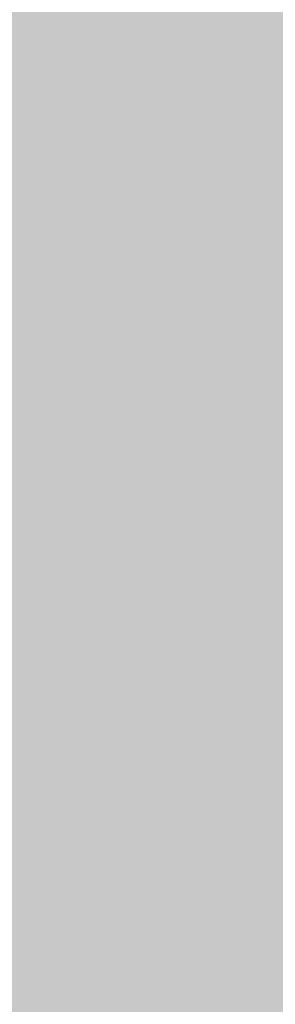
# Model space of a CAD drawing. Units: inches. Extents: x 2083 to 3317, y 1141 to 2115.
# Tile 216 of 256: x 3126.132 to 3126.67, y 1265.165 to 1267.234. Entities that reach past the tile are written whole.
import ezdxf

# ---------------------------------------------------------------- set-up
doc = ezdxf.new("R2010")
doc.units = ezdxf.units.IN
doc.layers.add('A-ANNO-DIMS', color=2, linetype='Continuous', lineweight=18)
doc.layers.add('A-WALL-PATT', color=251, linetype='Continuous', lineweight=13, true_color=0x636466)
doc.styles.get("Standard").update_dxf_attribs({"font": 'arial.ttf'})
doc.dimstyles.new('ISO-25', dxfattribs={"dimtxt": 12, "dimasz": 12, "dimexe": 1.25, "dimexo": 0.625, "dimtad": 1, "dimlunit": 3, "dimtxsty": 'Standard', "dimcen": 2.5, "dimadec": 0, "dimazin": 0, "dimtfac": 1, "dimtmove": 0, "dimatfit": 3, "dimfxl": 1, "dimarcsym": 0})

# ---------------------------------------------------------------- blocks, each defined once
blk = doc.blocks.new('*D26')
at = {"layer": 'A-ANNO-DIMS', "color": 0, "lineweight": -2, "transparency": 16777216}
for p, q in [((3088.9858, 1274.9151), (3088.9858, 1270.952)), ((3111.24, 1274.9151), (3111.24, 1270.952)), ((3076.9858, 1272.202), (2840.2624, 1272.202)), ((3111.24, 1272.202), (3088.9858, 1272.202)), ((3123.24, 1272.202), (3135.24, 1272.202))]:
    blk.add_line(p, q, dxfattribs=at)
at = {"layer": 'A-ANNO-DIMS', "color": 0, "transparency": 16777216}
for points in [[(3076.9858, 1274.202), (3076.9858, 1270.202), (3088.9858, 1272.202)], [(3123.24, 1274.202), (3123.24, 1270.202), (3111.24, 1272.202)]]:
    blk.add_solid(points, dxfattribs=at)
at = {"layer": 'Defpoints', "color": 0, "transparency": 16777216}
for p in [(3088.9858, 1275.5401), (3111.24, 1275.5401), (3088.9858, 1272.202)]:
    blk.add_point(p, dxfattribs=at)
at = {"layer": 'A-ANNO-DIMS', "color": 0, "transparency": 16777216, "insert": (2952.6241, 1279.0316), "char_height": 12, "attachment_point": 5}
blk.add_mtext('NIGHTSTAND 1\'-10 1/2" TYP.', dxfattribs=at)
blk = doc.blocks.new('*D27')
at = {"layer": 'A-ANNO-DIMS', "color": 0, "lineweight": -2, "transparency": 16777216}
for p, q in [((3114.5782, 1309.7943), (3114.5782, 1321.7943)), ((3111.865, 1297.7943), (3115.8282, 1297.7943)), ((3114.5782, 1297.7943), (3114.5782, 1275.5401)), ((3111.865, 1275.5401), (3115.8282, 1275.5401)), ((3114.5782, 1263.5401), (3114.5782, 1140.9886))]:
    blk.add_line(p, q, dxfattribs=at)
at = {"layer": 'A-ANNO-DIMS', "color": 0, "transparency": 16777216}
for points in [[(3112.5782, 1309.7943), (3116.5782, 1309.7943), (3114.5782, 1297.7943)], [(3112.5782, 1263.5401), (3116.5782, 1263.5401), (3114.5782, 1275.5401)]]:
    blk.add_solid(points, dxfattribs=at)
at = {"layer": 'Defpoints', "color": 0, "transparency": 16777216}
for p in [(3111.24, 1297.7943), (3111.24, 1275.5401), (3114.5782, 1275.5401)]:
    blk.add_point(p, dxfattribs=at)
at = {"layer": 'A-ANNO-DIMS', "color": 0, "transparency": 16777216, "insert": (3107.7485, 1196.2643), "char_height": 12, "attachment_point": 5, "rotation": 90}
blk.add_mtext('1\'-10 1/2" TYP.', dxfattribs=at)

msp = doc.modelspace()

# ---------------------------------------------------------------- hatches: boundary and pattern name
at = {"layer": 'A-WALL-PATT'}
h = msp.add_hatch(color=256, dxfattribs=at)
h.dxf.hatch_style = 1
h.paths.add_polyline_path([(3126.9598, 2020.7614), (2748.9598, 2020.7614), (2604.9598, 2020.7614), (2226.9598, 2020.7614), (2226.9598, 1702.7614), (2466.9598, 1702.7614), (2466.9598, 1582.7614), (2418.9598, 1582.7614), (2418.9598, 1477.7614), (2226.9598, 1477.7614), (2226.9598, 1263.2614), (2544.9598, 1263.2614), (2544.9598, 1411.7614), (2604.9598, 1411.7614), (2685.9598, 1411.7614), (2685.9598, 1420.7614), (2604.9598, 1420.7614), (2604.9598, 1573.7614), (2604.9598, 1702.7614), (2604.9598, 2011.7614), (2748.9598, 2011.7614), (2748.9598, 1702.7614), (2862.9598, 1702.7614), (2862.9598, 1621.7614), (2871.9598, 1621.7614), (2871.9598, 1702.7614), (2883.9598, 1702.7614), (2883.9598, 1706.9395, -0.026459), (2883.9598, 1711.7614), (2757.9598, 1711.7614), (2757.9598, 1807.7614), (2787.9598, 1807.7614), (2787.9598, 1812.2614), (2757.9598, 1812.2614), (2757.9598, 2011.7614), (2877.9598, 2011.7614), (2877.9598, 1812.2614), (2847.9598, 1812.2614), (2847.9598, 1807.7614), (2889.8357, 1807.7614), (2889.8357, 1812.2614), (2882.4598, 1812.2614), (2882.4598, 2011.7614), (3117.9598, 2011.7614), (3117.9598, 1812.2614), (2937.8357, 1812.2614), (2937.8357, 1807.7614), (2995.7098, 1807.7614), (2995.7098, 1796.1177), (3000.2098, 1796.1177), (3000.2098, 1807.7614), (3117.9598, 1807.7614), (3117.9598, 1711.7614), (3000.2098, 1711.7614), (3000.2098, 1760.1177), (2998.5727, 1760.1177, -0.020711), (2995.7098, 1760.1177), (2995.7098, 1711.7614), (2931.9598, 1711.7614), (2931.9598, 1702.7614), (3126.9598, 1702.7614)])
h.paths.add_polyline_path([(2471.4598, 2011.7614), (2471.4598, 1810.0114), (2462.7169, 1810.0114), (2462.7169, 1805.5114), (2505.9598, 1805.5114), (2505.9598, 1810.0114), (2475.9598, 1810.0114), (2475.9598, 2011.7614), (2595.9598, 2011.7614), (2595.9598, 1810.0114), (2565.9598, 1810.0114), (2565.9598, 1805.5114), (2595.9598, 1805.5114), (2595.9598, 1711.7614), (2235.9598, 1711.7614), (2235.9598, 1805.5114), (2353.7098, 1805.5114), (2353.7098, 1796.0542), (2358.2098, 1796.0542), (2358.2098, 1805.5114), (2414.7169, 1805.5114), (2414.7169, 1810.0114), (2235.9598, 1810.0114), (2235.9598, 2011.7614)], flags=16)
h.paths.add_polyline_path([(2270.2047, 1994.61), (2270.2047, 1970.61), (2246.2047, 1970.61), (2246.2047, 1994.61)], flags=0)
edge = h.paths.add_edge_path(flags=0)
edge.add_ellipse((2332.0274, 1899.7982), major_axis=(-3.043, 3.043), ratio=0.168252, start_angle=-161.3322, end_angle=-156.3071, ccw=False)
edge.add_ellipse((2333.082, 1898.7435), major_axis=(-1.0546, 1.0546), ratio=0.453532, start_angle=-123.371, end_angle=-94.1591)
edge = h.paths.add_edge_path(flags=0)
edge.add_ellipse((2332.0274, 1968.8763), major_axis=(3.043, 3.043), ratio=0.168252, start_angle=18.6678, end_angle=23.6929)
edge.add_spline(control_points=[(2332.9256, 1970.6911), (2332.2268, 1970.3361), (2330.8937, 1969.6589), (2328.4131, 1970.9321), (2327.2039, 1967.7487), (2324.7096, 1969.9556), (2322.5328, 1967.0124), (2320.0128, 1971.2958), (2317.6803, 1968.1578), (2316.0405, 1967.102), (2315.4269, 1966.8096)], knot_values=[0, 0, 0, 0, 2.267059, 4.324559, 6.685584, 8.878641, 11.121502, 14.300359, 17.755284, 19.732645, 19.732645, 19.732645, 19.732645], degree=3, periodic=0)
edge.add_ellipse((2332.0274, 1968.8763), major_axis=(3.043, 3.043), ratio=0.168252, start_angle=18.6678, end_angle=23.6929, ccw=False)
edge.add_ellipse((2333.082, 1969.9309), major_axis=(1.0546, 1.0546), ratio=0.453532, start_angle=56.629, end_angle=85.8409, ccw=False)
edge = h.paths.add_edge_path(flags=0)
edge.add_spline(control_points=[(2296.4283, 1967.9879), (2293.6278, 1965.3363), (2287.7036, 1959.7271), (2299.7439, 1949.9957), (2294.5326, 1935.6685), (2290.5732, 1920.6035), (2293.3941, 1909.9737), (2296.1854, 1904.9665)], knot_values=[0.099185, 0.099185, 0.099185, 0.099185, 0.345301, 0.619822, 0.982653, 1.386093, 1.810555, 1.810555, 1.810555, 1.810555], degree=3, periodic=0)
edge.add_spline(control_points=[(2296.1854, 1904.9665), (2297.3836, 1902.6193), (2298.001, 1901.9493), (2298.553, 1901.4682)], knot_values=[0.006246, 0.006246, 0.006246, 0.006246, 0.055476, 0.055476, 0.055476, 0.055476], degree=3, periodic=0)
edge.add_spline(control_points=[(2298.553, 1901.4682), (2297.2586, 1900.9232), (2295.2253, 1900.2321), (2293.0602, 1900.6142), (2292.1014, 1900.7884), (2292.0896, 1900.7906)], knot_values=[0.312835, 0.312835, 0.312835, 0.312835, 0.40178, 0.474987, 0.475903, 0.475903, 0.475903, 0.475903], degree=3, periodic=0)
edge.add_arc((2292.7936, 1904.6641), 3.937, 215.4209, 259.6982, ccw=False)
edge.add_spline(control_points=[(2289.5853, 1902.3823), (2289.4767, 1902.5351), (2289.3685, 1902.688), (2289.2609, 1902.8412)], knot_values=[0.102872, 0.102872, 0.102872, 0.102872, 0.116896, 0.116896, 0.116896, 0.116896], degree=3, periodic=0)
edge.add_spline(control_points=[(2289.2609, 1902.8412), (2288.6866, 1902.5502), (2287.64, 1902.0199), (2285.8813, 1901.874), (2283.853, 1901.5044), (2281.72, 1899.7105), (2278.467, 1899.4929), (2276.1571, 1901.8832), (2272.259, 1899.8041), (2267.7776, 1901.8432), (2262.2439, 1900.184), (2257.4149, 1901.7821), (2254.3184, 1900.7261), (2253.1783, 1900.3373)], knot_values=[0, 0, 0, 0, 1.907977, 3.477176, 5.261074, 7.972851, 11.680248, 13.717921, 16.939592, 22.789562, 27.502503, 33.595215, 37.145618, 37.145618, 37.145618, 37.145618], degree=3, periodic=0)
edge.add_line((2253.1783, 1900.3373), (2250.2442, 1902.8412))
edge.add_line((2250.2442, 1902.8412), (2250.2442, 1965.8333))
edge.add_line((2250.2442, 1965.8333), (2253.1783, 1968.3371))
edge.add_spline(control_points=[(2253.1783, 1968.3371), (2254.3184, 1967.9483), (2257.4149, 1966.8924), (2262.2439, 1968.4904), (2267.7776, 1966.8313), (2271.5267, 1968.5372), (2273.8759, 1967.8283), (2274.2067, 1967.7276)], knot_values=[0, 0, 0, 0, 0.09018, 0.244935, 0.364644, 0.513233, 0.537855, 0.537855, 0.537855, 0.537855], degree=3, periodic=0)
edge.add_arc((2274.3529, 1963.7933), 3.937, 72.0511, 92.1279, ccw=False)
edge.add_arc((2281.2969, 1985.23), 18.5963, 252.05113, 288.56572)
edge.add_arc((2292.3167, 1956.0289), 12.6461, 71.02679, 113.77822, ccw=False)
edge = h.paths.add_edge_path(flags=0)
edge.add_spline(control_points=[(2274.8994, 1951.8562), (2275.0662, 1951.6166), (2275.2327, 1951.3766), (2275.398, 1951.1359)], knot_values=[1.409916, 1.409916, 1.409916, 1.409916, 1.43159, 1.43159, 1.43159, 1.43159], degree=3, periodic=0)
edge.add_spline(control_points=[(2275.398, 1951.1359), (2275.7921, 1950.5619), (2276.1792, 1949.9838), (2276.5455, 1949.3971)], knot_values=[1.358238, 1.358238, 1.358238, 1.358238, 1.409916, 1.409916, 1.409916, 1.409916], degree=3, periodic=0)
edge.add_line((2276.5455, 1949.3971), (2277.4373, 1947.8622))
edge.add_spline(control_points=[(2277.4373, 1947.8622), (2276.3038, 1945.6731), (2274.6397, 1942.4269), (2274.6316, 1938.0939), (2272.7991, 1930.8515), (2274.3564, 1943.897), (2275.9477, 1947.9234), (2276.5455, 1949.3971)], knot_values=[0.005632, 0.005632, 0.005632, 0.005632, 0.186014, 0.266002, 0.357087, 0.59639, 0.739732, 0.739732, 0.739732, 0.739732], degree=3, periodic=0)
edge.add_spline(control_points=[(2276.5455, 1949.3971), (2276.1792, 1949.9838), (2275.7921, 1950.5619), (2275.398, 1951.1359)], knot_values=[1.358238, 1.358238, 1.358238, 1.358238, 1.409916, 1.409916, 1.409916, 1.409916], degree=3, periodic=0)
edge.add_spline(control_points=[(2275.398, 1951.1359), (2274.9425, 1950.0805), (2274.2078, 1948.0253), (2273.9346, 1944.8515), (2272.4685, 1937.6275), (2273.4662, 1945.6965), (2274.7006, 1951.0595), (2274.8994, 1951.8562)], knot_values=[0.104364, 0.104364, 0.104364, 0.104364, 0.189636, 0.269624, 0.36071, 0.600013, 0.644622, 0.644622, 0.644622, 0.644622], degree=3, periodic=0)
h.paths.add_polyline_path([(2269.1675, 1963.1276, -0.357527), (2268.1706, 1960.9764, -0.092561), (2268.1706, 1939.4363, -0.357527), (2269.1675, 1937.2851, -0.357527), (2267.0163, 1938.282, -0.164785), (2254.6856, 1938.282, -0.357527), (2252.5344, 1937.2851, -0.357527), (2253.5313, 1939.4363, -0.092561), (2253.5313, 1960.9764, -0.357527), (2252.5344, 1963.1276, -0.357527), (2254.6856, 1962.1307, -0.164785), (2267.0163, 1962.1307, -0.357527)], flags=0)
h.paths.add_polyline_path([(2248.8741, 1967.8018), (2248.8741, 1957.0277), (2249.4578, 1957.0277), (2249.4578, 1911.6468), (2248.8741, 1911.6468), (2248.8741, 1900.8727), (2246.5119, 1900.8727, 0.197327), (2244.1497, 1902.4569), (2244.1497, 1966.2176, 0.197327), (2246.5119, 1967.8018)], flags=0)
h.paths.add_polyline_path([(2269.1675, 1931.3893, -0.357527), (2268.1706, 1929.2381, -0.092561), (2268.1706, 1907.6981, -0.357527), (2269.1675, 1905.5469, -0.357527), (2267.0163, 1906.5438, -0.164785), (2254.6856, 1906.5438, -0.357527), (2252.5344, 1905.5469, -0.357527), (2253.5313, 1907.6981, -0.092561), (2253.5313, 1929.2381, -0.357527), (2252.5344, 1931.3893, -0.357527), (2254.6856, 1930.3925, -0.164785), (2267.0163, 1930.3925, -0.357527)], flags=0)
edge = h.paths.add_edge_path(flags=0)
edge.add_spline(control_points=[(2276.1969, 1906.7237), (2276.1681, 1909.0289), (2276.114, 1913.3719), (2270.5984, 1924.925), (2273.9052, 1919.0128), (2275.9217, 1916.2621), (2275.4746, 1912.4021), (2277.2579, 1910.3806), (2276.696, 1908.225), (2276.6462, 1906.813), (2276.6178, 1906.0084)], knot_values=[0, 0, 0, 0, 8.61026, 16.221274, 18.843057, 23.804898, 27.440828, 29.356102, 31.203478, 33.650687, 33.650687, 33.650687, 33.650687], degree=3, periodic=0)
edge.add_spline(control_points=[(2276.6178, 1906.0084), (2276.6233, 1905.6241), (2276.4977, 1904.6287), (2275.4418, 1903.8547), (2274.9373, 1903.0804), (2274.8591, 1902.8412)], knot_values=[0.156488, 0.156488, 0.156488, 0.156488, 0.184398, 0.231376, 0.250598, 0.250598, 0.250598, 0.250598], degree=3, periodic=0)
edge.add_line((2274.8591, 1902.8412), (2276.506, 1902.8412))
edge.add_spline(control_points=[(2276.506, 1902.8412), (2276.7883, 1903.0849), (2277.6651, 1904.1252), (2278.2495, 1904.3407), (2277.6539, 1908.5274), (2278.1557, 1906.2278), (2278.1005, 1905.2859), (2278.8467, 1904.069), (2277.8568, 1903.4149), (2277.8742, 1902.991), (2277.9036, 1902.8412)], knot_values=[0.059574, 0.059574, 0.059574, 0.059574, 0.080753, 0.103741, 0.16972, 0.176036, 0.207137, 0.240474, 0.262341, 0.27366, 0.27366, 0.27366, 0.27366], degree=3, periodic=0)
edge.add_line((2277.9036, 1902.8412), (2280.0298, 1902.8412))
edge.add_spline(control_points=[(2280.0298, 1902.8412), (2279.8882, 1903.0884), (2279.4993, 1903.9816), (2280.1523, 1905.9393), (2278.1036, 1909.6578), (2279.7624, 1907.1853), (2280.3279, 1904.8749), (2280.4851, 1903.4896), (2281.4633, 1903.2494), (2281.7583, 1902.9365), (2281.834, 1902.8412)], knot_values=[0.013856, 0.013856, 0.013856, 0.013856, 0.034874, 0.088867, 0.107879, 0.126738, 0.158714, 0.193757, 0.217487, 0.226722, 0.226722, 0.226722, 0.226722], degree=3, periodic=0)
edge.add_spline(control_points=[(2281.834, 1902.8412), (2281.7875, 1902.8267), (2281.647, 1902.783), (2281.3955, 1902.8595), (2281.0881, 1902.9852), (2280.7207, 1903.0609), (2280.3335, 1903.0257), (2280.1248, 1902.8989), (2280.0298, 1902.8412)], knot_values=[0, 0, 0, 0, 0.14413, 0.435517, 0.749276, 1.153046, 1.548371, 1.878348, 1.878348, 1.878348, 1.878348], degree=3, periodic=0)
edge.add_line((2280.0298, 1902.8412), (2277.9036, 1902.8412))
edge.add_spline(control_points=[(2277.9036, 1902.8412), (2277.8929, 1902.7959), (2277.8654, 1902.6796), (2277.6075, 1902.6875), (2277.2741, 1902.8007), (2276.8379, 1902.6198), (2276.5838, 1902.7893), (2276.506, 1902.8412)], knot_values=[0, 0, 0, 0, 0.127189, 0.326199, 0.628009, 1.24357, 1.515331, 1.515331, 1.515331, 1.515331], degree=3, periodic=0)
edge.add_line((2276.506, 1902.8412), (2274.8591, 1902.8412))
edge.add_spline(control_points=[(2274.8591, 1902.8412), (2274.8144, 1902.8986), (2274.7251, 1903.0134), (2274.4935, 1903.119), (2274.2443, 1902.9605), (2273.9371, 1903.1849), (2273.614, 1902.9831), (2273.4083, 1902.883), (2273.3223, 1902.8412)], knot_values=[0, 0, 0, 0, 0.21843, 0.436957, 0.687977, 0.990379, 1.398396, 1.69185, 1.69185, 1.69185, 1.69185], degree=3, periodic=0)
edge.add_spline(control_points=[(2273.3223, 1902.8412), (2273.6167, 1903.4457), (2274.274, 1904.5383), (2276.0272, 1904.5737), (2276.207, 1906.5836), (2276.1969, 1906.7237)], knot_values=[0.012227, 0.012227, 0.012227, 0.012227, 0.059472, 0.106218, 0.134458, 0.134458, 0.134458, 0.134458], degree=3, periodic=0)
h.paths.add_polyline_path([(2270.7761, 1897.7898), (2270.7761, 1873.7898), (2246.7761, 1873.7898), (2246.7761, 1897.7898)], flags=0)
h.paths.add_polyline_path([(2353.7098, 1760.0051), (2353.7098, 1760.0542), (2358.2098, 1760.0542, -0.033729)], flags=0)
h.paths.add_polyline_path([(2321.8191, 1737.5292), (2341.9953, 1737.5292, -0.414214), (2343.2033, 1736.3212), (2343.2033, 1721.0206, -0.414214), (2341.9953, 1719.8127), (2321.8191, 1719.8127, -0.414214), (2320.6112, 1721.0206), (2320.6112, 1736.3212, -0.414214)], flags=0)
h.paths.add_polyline_path([(2324.235, 1736.3212), (2339.5794, 1736.3212, -0.414214), (2341.9953, 1733.9053), (2341.9953, 1725.4497, -0.414214), (2339.5794, 1723.0338), (2333.6806, 1723.0338), (2333.8453, 1722.0455, -0.870646), (2335.4254, 1721.8259, -0.767327), (2333.9227, 1721.4232), (2331.291, 1721.4232, -0.767327), (2329.7883, 1721.8259, -0.870646), (2331.3684, 1722.0455), (2331.5331, 1723.0338), (2324.235, 1723.0338, -0.414214), (2321.8191, 1725.4497), (2321.8191, 1733.9053, -0.414214)], flags=0)
h.paths.add_polyline_path([(2570.4838, 1928.6154), (2589.6838, 1928.6154), (2590.1688, 1928.6154), (2590.1688, 1904.9934), (2570.4838, 1904.9934)], flags=0)
h.paths.add_polyline_path([(2574.4473, 1927.2638, -1), (2572.8288, 1927.2638, -1)], flags=0)
h.paths.add_polyline_path([(2573.0899, 1926.9409), (2573.925, 1927.776), (2574.1477, 1927.5533), (2573.3126, 1926.7182)], flags=0)
h.paths.add_polyline_path([(2578.7791, 1919.7296, -1), (2571.5917, 1919.7296, -1)], flags=0)
h.paths.add_polyline_path([(2578.3854, 1919.7296, -1), (2571.9854, 1919.7296, -1)], flags=0)
h.paths.add_polyline_path([(2331.5958, 1729.4762, -1), (2333.618, 1729.4762, -1)], flags=0)
h.paths.add_polyline_path([(2578.0342, 1927.2638, -1), (2576.4157, 1927.2638, -1)], flags=0)
h.paths.add_polyline_path([(2576.6889, 1927.5311), (2576.9116, 1927.7538), (2577.7467, 1926.9186), (2577.524, 1926.6959)], flags=0)
h.paths.add_polyline_path([(2578.1391, 1909.8595, -1), (2572.2317, 1909.8595, -1)], flags=0)
h.paths.add_polyline_path([(2577.7454, 1909.8595, -1), (2572.6254, 1909.8595, -1)], flags=0)
h.paths.add_polyline_path([(2583.7977, 1927.2638, -1), (2582.1792, 1927.2638, -1)], flags=0)
h.paths.add_polyline_path([(2582.7186, 1927.7538), (2583.5538, 1926.9186), (2583.3311, 1926.6959), (2582.4959, 1927.5311)], flags=0)
h.paths.add_polyline_path([(2582.4959, 1927.5311), (2582.7186, 1927.7538), (2583.5538, 1926.9186), (2583.3311, 1926.6959)], flags=0)
h.paths.add_polyline_path([(2587.7391, 1920.5296, -1), (2581.8317, 1920.5296, -1)], flags=0)
h.paths.add_polyline_path([(2587.3454, 1920.5296, -1), (2582.2254, 1920.5296, -1)], flags=0)
h.paths.add_polyline_path([(2587.3846, 1927.2638, -1), (2585.7661, 1927.2638, -1)], flags=0)
h.paths.add_polyline_path([(2586.082, 1926.9802), (2586.9172, 1927.8154), (2587.1399, 1927.5927), (2586.3047, 1926.7575)], flags=0)
h.paths.add_polyline_path([(2588.3791, 1910.6595, -1), (2581.1917, 1910.6595, -1)], flags=0)
h.paths.add_polyline_path([(2587.9854, 1910.6595, -1), (2581.5854, 1910.6595, -1)], flags=0)
h.paths.add_polyline_path([(2417.1677, 1729.4779), (2437.3439, 1729.4779, -0.414214), (2438.5519, 1728.2699), (2438.5519, 1712.9693, -0.414214), (2437.3439, 1711.7614), (2417.1677, 1711.7614, -0.414214), (2415.9598, 1712.9693), (2415.9598, 1728.2699, -0.414214)], flags=0)
h.paths.add_polyline_path([(2419.5836, 1728.2699), (2434.928, 1728.2699, -0.414214), (2437.3439, 1725.8541), (2437.3439, 1717.3984, -0.414214), (2434.928, 1714.9825), (2429.0292, 1714.9825), (2429.1939, 1713.9942, -0.870646), (2430.774, 1713.7746, -0.767327), (2429.2713, 1713.372), (2426.6396, 1713.372, -0.767327), (2425.1369, 1713.7746, -0.870646), (2426.717, 1713.9942), (2426.8817, 1714.9825), (2419.5836, 1714.9825, -0.414214), (2417.1677, 1717.3984), (2417.1677, 1725.8541, -0.414214)], flags=0)
h.paths.add_polyline_path([(2419.5836, 1728.2699), (2434.928, 1728.2699, -0.414214), (2437.3439, 1725.8541), (2437.3439, 1717.3984, -0.414214), (2434.928, 1714.9825), (2429.0292, 1714.9825), (2428.3581, 1719.009), (2427.5528, 1719.009), (2426.8817, 1714.9825), (2419.5836, 1714.9825, -0.414214), (2417.1677, 1717.3984), (2417.1677, 1725.8541, -0.414214)], flags=0)
h.paths.add_polyline_path([(2426.9444, 1721.4249, -1), (2428.9666, 1721.4249, -1)], flags=0)
h.paths.add_polyline_path([(2475.9598, 1702.7614), (2595.9598, 1702.7614), (2595.9598, 1582.7614), (2475.9598, 1582.7614)], flags=16)
h.paths.add_polyline_path([(2427.9598, 1573.7614), (2595.9598, 1573.7614), (2595.9598, 1468.7614), (2595.9598, 1420.7614), (2384.4598, 1420.7614), (2384.4598, 1468.7614), (2427.9598, 1468.7614)], flags=16)
h.paths.add_polyline_path([(2379.9598, 1468.7614), (2379.9598, 1420.7614), (2235.9598, 1420.7614), (2235.9598, 1468.7614)], flags=16)
h.paths.add_polyline_path([(2317.816, 1466.6958), (2337.9922, 1466.6958, -0.414214), (2339.2002, 1465.4878), (2339.2002, 1450.1872, -0.414214), (2337.9922, 1448.9792), (2317.816, 1448.9792, -0.414214), (2316.6081, 1450.1872), (2316.6081, 1465.4878, -0.414214)], flags=0)
h.paths.add_polyline_path([(2320.2319, 1465.4878), (2335.5763, 1465.4878, -0.414214), (2337.9922, 1463.0719), (2337.9922, 1454.6163, -0.414214), (2335.5763, 1452.2004), (2329.6775, 1452.2004), (2329.8422, 1451.212, -0.870646), (2331.4223, 1450.9925, -0.767327), (2329.9196, 1450.5898), (2327.2879, 1450.5898, -0.767327), (2325.7852, 1450.9925, -0.870646), (2327.3653, 1451.212), (2327.53, 1452.2004), (2320.2319, 1452.2004, -0.414214), (2317.816, 1454.6163), (2317.816, 1463.0719, -0.414214)], flags=0)
h.paths.add_polyline_path([(2320.2319, 1465.4878), (2335.5763, 1465.4878, -0.414214), (2337.9922, 1463.0719), (2337.9922, 1454.6163, -0.414214), (2335.5763, 1452.2004), (2329.6775, 1452.2004), (2329.0064, 1456.2269), (2328.2011, 1456.2269), (2327.53, 1452.2004), (2320.2319, 1452.2004, -0.414214), (2317.816, 1454.6163), (2317.816, 1463.0719, -0.414214)], flags=0)
h.paths.add_polyline_path([(2327.5926, 1458.6428, -1), (2329.6148, 1458.6428, -1)], flags=0)
h.paths.add_polyline_path([(2244.4117, 1433.3405), (2241.9209, 1433.3405, -0.414214), (2240.0179, 1435.2435), (2240.0179, 1440.9528, -0.414211), (2241.9209, 1442.8559), (2244.4117, 1442.8559, -1.976472)], flags=0)
h.paths.add_polyline_path([(2245.3569, 1434.3975, -0.414214), (2245.3569, 1441.7988, -2.144098)], flags=0)
h.paths.add_polyline_path([(2535.9598, 1416.2614), (2535.9598, 1272.2614), (2235.9598, 1272.2614), (2235.9598, 1416.2614)], flags=16)
h.paths.add_polyline_path([(2260.1196, 1384.2928), (2260.1196, 1362.0386), (2237.8654, 1362.0386), (2237.8654, 1384.2928)], flags=0)
edge = h.paths.add_edge_path(flags=0)
edge.add_line((2318.2518, 1362.0933), (2318.1458, 1362.001))
edge.add_ellipse((2317.4451, 1360.431), major_axis=(2.8216, 2.8216), ratio=0.168252, start_angle=18.6678, end_angle=20.9481, ccw=False)
edge.add_ellipse((2318.423, 1361.409), major_axis=(0.9779, 0.9779), ratio=0.453532, start_angle=56.629, end_angle=70.2262, ccw=False)
edge = h.paths.add_edge_path(flags=0)
edge.add_line((2319.1074, 1295.5711), (2319.015, 1295.6771))
edge.add_ellipse((2317.4451, 1296.3778), major_axis=(-2.8216, 2.8216), ratio=0.168252, start_angle=-161.3322, end_angle=-159.0519, ccw=False)
edge.add_ellipse((2318.423, 1295.3999), major_axis=(-0.9779, 0.9779), ratio=0.453532, start_angle=-123.371, end_angle=-109.7738)
edge = h.paths.add_edge_path(flags=0)
edge.add_spline(control_points=[(2284.2103, 1301.1702), (2284.5807, 1300.4447), (2284.8912, 1299.892), (2285.1596, 1299.461)], knot_values=[0.039066, 0.039066, 0.039066, 0.039066, 0.055476, 0.055476, 0.055476, 0.055476], degree=3, periodic=0)
edge.add_line((2285.1596, 1299.461), (2284.2103, 1301.1702))
edge = h.paths.add_edge_path(flags=0)
edge.add_line((2280.4125, 1297.298), (2283.37, 1297.0361))
edge.add_line((2283.37, 1297.0361), (2286.4057, 1297.9263))
edge.add_spline(control_points=[(2286.4057, 1297.9263), (2285.3055, 1297.4631), (2284.3448, 1297.1292), (2283.37, 1297.0361)], knot_values=[0.394369, 0.394369, 0.394369, 0.394369, 0.475903, 0.475903, 0.475903, 0.475903], degree=3, periodic=0)
edge.add_spline(control_points=[(2283.37, 1297.0361), (2283.2814, 1297.0277), (2282.3163, 1296.9573), (2281.3125, 1297.1345), (2280.4234, 1297.296), (2280.4125, 1297.298)], knot_values=[0.312835, 0.312835, 0.312835, 0.312835, 0.320246, 0.393453, 0.394369, 0.394369, 0.394369, 0.394369], degree=3, periodic=0)
edge = h.paths.add_edge_path(flags=0)
edge.add_line((2284.4356, 1359.6073), (2280.4463, 1355.328))
edge.add_line((2280.4463, 1355.328), (2279.58, 1351.0178))
edge.add_line((2279.58, 1351.0178), (2282.413, 1346.5804))
edge.add_spline(control_points=[(2282.413, 1346.5804), (2283.1533, 1345.5892), (2284.2529, 1344.0289), (2284.801, 1342.3872), (2284.9352, 1341.8055)], knot_values=[1.240098, 1.240098, 1.240098, 1.240098, 1.332892, 1.382712, 1.382712, 1.382712, 1.382712], degree=3, periodic=0)
edge.add_spline(control_points=[(2284.9352, 1341.8055), (2285.3191, 1340.1406), (2285.233, 1338.4092), (2284.9099, 1336.6541)], knot_values=[1.097484, 1.097484, 1.097484, 1.097484, 1.240098, 1.240098, 1.240098, 1.240098], degree=3, periodic=0)
edge.add_spline(control_points=[(2284.9099, 1336.6541), (2284.5868, 1334.899), (2284.0267, 1333.1203), (2283.4626, 1331.3606)], knot_values=[0.95487, 0.95487, 0.95487, 0.95487, 1.097484, 1.097484, 1.097484, 1.097484], degree=3, periodic=0)
edge.add_line((2283.4626, 1331.3606), (2281.8904, 1326.1534))
edge.add_line((2281.8904, 1326.1534), (2280.7563, 1321.0561))
edge.add_line((2280.7563, 1321.0561), (2280.2992, 1316.002))
edge.add_line((2280.2992, 1316.002), (2280.7159, 1310.9501))
edge.add_line((2280.7159, 1310.9501), (2282.0281, 1305.9721))
edge.add_line((2282.0281, 1305.9721), (2284.2103, 1301.1702))
edge.add_spline(control_points=[(2284.2103, 1301.1702), (2283.3407, 1302.7302), (2282.6119, 1304.3365), (2282.0281, 1305.9721)], knot_values=[0.099185, 0.099185, 0.099185, 0.099185, 0.241799, 0.241799, 0.241799, 0.241799], degree=3, periodic=0)
edge.add_spline(control_points=[(2282.0281, 1305.9721), (2281.4443, 1307.6078), (2281.0055, 1309.2728), (2280.7159, 1310.9501)], knot_values=[0.241799, 0.241799, 0.241799, 0.241799, 0.384413, 0.384413, 0.384413, 0.384413], degree=3, periodic=0)
edge.add_spline(control_points=[(2280.7159, 1310.9501), (2280.4332, 1312.5876), (2280.2894, 1314.277), (2280.2989, 1315.962), (2280.2992, 1316.002)], knot_values=[0.384413, 0.384413, 0.384413, 0.384413, 0.523647, 0.527028, 0.527028, 0.527028, 0.527028], degree=3, periodic=0)
edge.add_spline(control_points=[(2280.2992, 1316.002), (2280.3123, 1317.687), (2280.4779, 1319.3679), (2280.7563, 1321.0561)], knot_values=[0.527028, 0.527028, 0.527028, 0.527028, 0.669642, 0.669642, 0.669642, 0.669642], degree=3, periodic=0)
edge.add_spline(control_points=[(2280.7563, 1321.0561), (2281.0346, 1322.7443), (2281.4259, 1324.4396), (2281.8904, 1326.1534)], knot_values=[0.669642, 0.669642, 0.669642, 0.669642, 0.812256, 0.812256, 0.812256, 0.812256], degree=3, periodic=0)
edge.add_spline(control_points=[(2281.8904, 1326.1534), (2282.2644, 1327.5333), (2282.7879, 1329.2618), (2283.3528, 1331.0178), (2283.4626, 1331.3606)], knot_values=[0.812256, 0.812256, 0.812256, 0.812256, 0.927087, 0.95487, 0.95487, 0.95487, 0.95487], degree=3, periodic=0)
edge.add_line((2283.4626, 1331.3606), (2284.9099, 1336.6541))
edge.add_line((2284.9099, 1336.6541), (2284.9352, 1341.8055))
edge.add_line((2284.9352, 1341.8055), (2282.413, 1346.5804))
edge.add_spline(control_points=[(2282.413, 1346.5804), (2281.2751, 1348.1038), (2280.0784, 1349.5703), (2279.58, 1351.0178)], knot_values=[1.382712, 1.382712, 1.382712, 1.382712, 1.525326, 1.525326, 1.525326, 1.525326], degree=3, periodic=0)
edge.add_spline(control_points=[(2279.58, 1351.0178), (2279.4433, 1351.4147), (2279.1363, 1352.8569), (2279.7352, 1354.2904), (2280.4463, 1355.328)], knot_values=[1.525326, 1.525326, 1.525326, 1.525326, 1.564439, 1.667941, 1.667941, 1.667941, 1.667941], degree=3, periodic=0)
edge.add_spline(control_points=[(2280.4463, 1355.328), (2281.4261, 1356.7578), (2282.9308, 1358.1826), (2284.4356, 1359.6073)], knot_values=[1.667941, 1.667941, 1.667941, 1.667941, 1.810555, 1.810555, 1.810555, 1.810555], degree=3, periodic=0)
edge.add_arc((2280.6231, 1348.5182), 11.7262, 71.02679, 113.77822)
edge.add_arc((2270.4049, 1375.5952), 17.2436, 252.05113, 288.56572, ccw=False)
edge.add_arc((2263.966, 1355.7178), 3.6506, 72.0511, 92.1279)
edge.add_arc((2263.966, 1355.7178), 3.6506, 92.1279, 177.9851)
edge.add_spline(control_points=[(2260.3176, 1355.8462), (2260.2604, 1354.2207), (2260.5513, 1350.1865), (2262.9993, 1346.7663), (2264.4727, 1344.649)], knot_values=[1.43159, 1.43159, 1.43159, 1.43159, 1.564144, 1.770695, 1.770695, 1.770695, 1.770695], degree=3, periodic=0)
edge.add_line((2264.4727, 1344.649), (2264.9356, 1343.9825))
edge.add_spline(control_points=[(2263.801, 1340.2481), (2263.8432, 1340.5141), (2264.0672, 1341.7565), (2264.5127, 1343.0025), (2264.935, 1343.9811)], knot_values=[0.53657, 0.53657, 0.53657, 0.53657, 0.559349, 0.644622, 0.644622, 0.644622, 0.644622], degree=3, periodic=0)
edge.add_spline(control_points=[(2264.935, 1343.9811), (2265.1178, 1343.715), (2265.2989, 1343.4479), (2265.4768, 1343.1794)], knot_values=[1.384077, 1.384077, 1.384077, 1.384077, 1.409916, 1.409916, 1.409916, 1.409916], degree=3, periodic=0)
edge.add_spline(control_points=[(2265.4768, 1343.1794), (2265.6546, 1342.9108), (2265.8293, 1342.6408), (2265.9991, 1342.3688)], knot_values=[1.358238, 1.358238, 1.358238, 1.358238, 1.384077, 1.384077, 1.384077, 1.384077], degree=3, periodic=0)
edge.add_line((2265.9991, 1342.3688), (2266.826, 1340.9455))
edge.add_spline(control_points=[(2266.826, 1340.9455), (2268.8944, 1337.0897), (2271.3982, 1325.843), (2270.5162, 1310.5686), (2275.9194, 1301.8606), (2277.7895, 1299.1994)], knot_values=[0.116896, 0.116896, 0.116896, 0.116896, 0.472987, 1.050969, 1.313793, 1.313793, 1.313793, 1.313793], degree=3, periodic=0)
edge.add_spline(control_points=[(2277.7895, 1299.1994), (2277.8394, 1299.1285), (2277.8894, 1299.0575), (2277.9396, 1298.9866)], knot_values=[0.109884, 0.109884, 0.109884, 0.109884, 0.116896, 0.116896, 0.116896, 0.116896], degree=3, periodic=0)
edge.add_line((2277.9396, 1298.9866), (2277.7888, 1299.1991))
edge.add_spline(control_points=[(2277.7888, 1299.1991), (2277.2566, 1298.9294), (2276.2864, 1298.4379), (2275.0394, 1298.3344), (2274.3833, 1298.2389), (2274.2153, 1298.2093)], knot_values=[33.12187, 33.12187, 33.12187, 33.12187, 35.029056, 36.598255, 37.144827, 37.144827, 37.144827, 37.144827], degree=3, periodic=0)
edge.add_line((2274.2153, 1298.2093), (2273.0731, 1297.893))
edge.add_spline(control_points=[(2273.0731, 1297.893), (2272.3229, 1297.5798), (2271.0392, 1296.5105), (2269.2484, 1296.2261), (2268.4231, 1296.3747)], knot_values=[26.532584, 26.532584, 26.532584, 26.532584, 29.198919, 31.839101, 31.839101, 31.839101, 31.839101], degree=3, periodic=0)
edge.add_line((2268.4231, 1296.3747), (2263.8785, 1297.4575))
edge.add_spline(control_points=[(2263.8785, 1297.4575), (2263.5561, 1297.3594), (2261.8603, 1296.8387), (2260.2388, 1297.2824), (2258.9335, 1297.5165)], knot_values=[15.919551, 15.919551, 15.919551, 15.919551, 16.939592, 21.226067, 21.226067, 21.226067, 21.226067], degree=3, periodic=0)
edge.add_line((2258.9335, 1297.5165), (2254.0552, 1297.329))
edge.add_spline(control_points=[(2254.0552, 1297.329), (2253.7555, 1297.2958), (2252.1137, 1297.1652), (2250.4619, 1297.5442), (2249.1297, 1297.6679)], knot_values=[5.306517, 5.306517, 5.306517, 5.306517, 6.276435, 10.613034, 10.613034, 10.613034, 10.613034], degree=3, periodic=0)
edge.add_line((2249.1297, 1297.6679), (2244.3316, 1296.8778))
edge.add_line((2244.3316, 1296.8778), (2241.611, 1299.1994))
edge.add_line((2241.611, 1299.1994), (2241.611, 1357.6094))
edge.add_line((2241.611, 1357.6094), (2244.3316, 1359.9311))
edge.add_line((2244.3316, 1359.9311), (2252.7288, 1359.5427))
edge.add_spline(control_points=[(2252.7288, 1359.5427), (2252.8709, 1359.5464), (2253.3057, 1359.5482), (2253.7398, 1359.5143), (2254.0317, 1359.4824)], knot_values=[0.233291, 0.233291, 0.233291, 0.233291, 0.244935, 0.268927, 0.268927, 0.268927, 0.268927], degree=3, periodic=0)
edge.add_line((2254.0317, 1359.4824), (2259.5872, 1359.4164))
edge.add_spline(control_points=[(2259.5872, 1359.4164), (2260.6771, 1359.6285), (2262.0732, 1359.897), (2263.5237, 1359.4593), (2263.8304, 1359.366)], knot_values=[0.422516, 0.422516, 0.422516, 0.422516, 0.513233, 0.537855, 0.537855, 0.537855, 0.537855], degree=3, periodic=0)
edge.add_arc((2263.966, 1355.7178), 3.6506, 72.0511, 92.1279, ccw=False)
edge.add_arc((2270.4049, 1375.5952), 17.2436, 252.05113, 288.56572)
edge.add_arc((2280.6231, 1348.5182), 11.7262, 71.02679, 113.77822, ccw=False)
h.paths.add_polyline_path([(2240.3405, 1359.4347), (2240.3405, 1349.4444), (2240.8818, 1349.4444), (2240.8818, 1307.3645), (2240.3405, 1307.3645), (2240.3405, 1297.3741), (2238.1502, 1297.3741, 0.197327), (2235.9598, 1298.8431), (2235.9598, 1357.9657, 0.197327), (2238.1502, 1359.4347)], flags=0)
h.paths.add_polyline_path([(2259.1578, 1355.1005, -0.357527), (2258.2334, 1353.1058, -0.092561), (2258.2334, 1333.1326, -0.357527), (2259.1578, 1331.1379, -0.357527), (2257.1631, 1332.0622, -0.164785), (2245.7293, 1332.0622, -0.357527), (2243.7346, 1331.1379, -0.357527), (2244.6589, 1333.1326, -0.092561), (2244.6589, 1353.1058, -0.357527), (2243.7346, 1355.1005, -0.357527), (2245.7293, 1354.1761, -0.164785), (2257.1631, 1354.1761, -0.357527)], flags=0)
edge = h.paths.add_edge_path(flags=0)
edge.add_line((2265.9991, 1342.3688), (2266.826, 1340.9455))
edge.add_line((2266.826, 1340.9455), (2265.3076, 1337.8141))
edge.add_line((2265.3076, 1337.8141), (2264.3582, 1334.6529))
edge.add_line((2264.3582, 1334.6529), (2264.262, 1333.7997))
edge.add_spline(control_points=[(2264.262, 1333.7997), (2264.2084, 1333.1871), (2264.1621, 1332.3655), (2264.0071, 1331.4139), (2263.969, 1331.2018)], knot_values=[0.464444, 0.464444, 0.464444, 0.464444, 0.516691, 0.531608, 0.531608, 0.531608, 0.531608], degree=3, periodic=0)
edge.add_spline(control_points=[(2263.969, 1331.2018), (2263.7745, 1330.1189), (2263.4244, 1328.7908), (2263.2574, 1328.5307), (2263.234, 1328.5146)], knot_values=[0.372682, 0.372682, 0.372682, 0.372682, 0.44885, 0.464444, 0.464444, 0.464444, 0.464444], degree=3, periodic=0)
edge.add_spline(control_points=[(2263.234, 1328.5146), (2263.0964, 1328.4202), (2263.1312, 1329.3015), (2263.275, 1330.6157)], knot_values=[0.280919, 0.280919, 0.280919, 0.280919, 0.372682, 0.372682, 0.372682, 0.372682], degree=3, periodic=0)
edge.add_spline(control_points=[(2263.275, 1330.6157), (2263.4187, 1331.93), (2263.6715, 1333.6773), (2263.9699, 1335.315)], knot_values=[0.189157, 0.189157, 0.189157, 0.189157, 0.280919, 0.280919, 0.280919, 0.280919], degree=3, periodic=0)
edge.add_spline(control_points=[(2263.9699, 1335.315), (2264.1005, 1336.0322), (2264.4188, 1337.6219), (2264.7548, 1338.8644), (2264.9474, 1339.4911)], knot_values=[0.097394, 0.097394, 0.097394, 0.097394, 0.137578, 0.189157, 0.189157, 0.189157, 0.189157], degree=3, periodic=0)
edge.add_spline(control_points=[(2264.9474, 1339.4911), (2265.29, 1340.6061), (2265.6442, 1341.494), (2265.9991, 1342.3688)], knot_values=[0.005632, 0.005632, 0.005632, 0.005632, 0.097394, 0.097394, 0.097394, 0.097394], degree=3, periodic=0)
h.paths.add_polyline_path([(2259.1578, 1325.671, -0.357527), (2258.2334, 1323.6763, -0.092561), (2258.2334, 1303.7031, -0.357527), (2259.1578, 1301.7084, -0.357527), (2257.1631, 1302.6327, -0.164785), (2245.7293, 1302.6327, -0.357527), (2243.7346, 1301.7084, -0.357527), (2244.6589, 1303.7031, -0.092561), (2244.6589, 1323.6763, -0.357527), (2243.7346, 1325.671, -0.357527), (2245.7293, 1324.7466, -0.164785), (2257.1631, 1324.7466, -0.357527)], flags=0)
edge = h.paths.add_edge_path(flags=0)
edge.add_spline(control_points=[(2261.7089, 1317.3114), (2261.6795, 1317.4176), (2261.7619, 1317.3885), (2262.4907, 1316.0899), (2262.9622, 1315.3009)], knot_values=[14.955861, 14.955861, 14.955861, 14.955861, 16.221274, 18.694826, 18.694826, 18.694826, 18.694826], degree=3, periodic=0)
edge.add_spline(control_points=[(2262.9622, 1315.3009), (2262.9904, 1315.2536), (2263.7021, 1314.0674), (2264.349, 1313.1272), (2264.7301, 1312.1642)], knot_values=[18.694826, 18.694826, 18.694826, 18.694826, 18.843057, 22.433791, 22.433791, 22.433791, 22.433791], degree=3, periodic=0)
edge.add_spline(control_points=[(2264.7301, 1312.1642), (2264.8756, 1311.7964), (2265.1769, 1310.7698), (2265.1431, 1309.5593), (2265.2477, 1308.8242)], knot_values=[22.433791, 22.433791, 22.433791, 22.433791, 23.804898, 26.172756, 26.172756, 26.172756, 26.172756], degree=3, periodic=0)
edge.add_line((2265.2477, 1308.8242), (2265.8508, 1307.1719))
edge.add_spline(control_points=[(2265.8508, 1307.1719), (2266.065, 1306.8217), (2266.3844, 1306.3322), (2266.4244, 1305.7805), (2266.4204, 1305.6112)], knot_values=[28.062562, 28.062562, 28.062562, 28.062562, 29.356102, 29.911721, 29.911721, 29.911721, 29.911721], degree=3, periodic=0)
edge.add_spline(control_points=[(2266.4204, 1305.6112), (2266.4161, 1305.4326), (2266.394, 1305.25), (2266.3648, 1305.0659)], knot_values=[29.911721, 29.911721, 29.911721, 29.911721, 30.497837, 30.497837, 30.497837, 30.497837], degree=3, periodic=0)
edge.add_line((2266.3648, 1305.0659), (2266.0662, 1302.1363))
edge.add_spline(control_points=[(2266.0662, 1302.1363), (2266.0712, 1301.78), (2265.9981, 1301.2), (2265.6633, 1300.759), (2265.5089, 1300.5859)], knot_values=[0.156488, 0.156488, 0.156488, 0.156488, 0.184398, 0.203543, 0.203543, 0.203543, 0.203543], degree=3, periodic=0)
edge.add_line((2265.5089, 1300.5859), (2264.4353, 1299.1994))
edge.add_line((2264.4353, 1299.1994), (2265.9624, 1299.1994))
edge.add_line((2265.9624, 1299.1994), (2267.336, 1301.1753))
edge.add_line((2267.336, 1301.1753), (2267.3117, 1301.9862))
edge.add_spline(control_points=[(2267.3117, 1301.9862), (2267.2611, 1302.8624), (2267.1602, 1303.7371), (2267.2715, 1303.3259)], knot_values=[0.126229, 0.126229, 0.126229, 0.126229, 0.166617, 0.166617, 0.166617, 0.166617], degree=3, periodic=0)
edge.add_spline(control_points=[(2267.2715, 1303.3259), (2267.28, 1303.2943), (2267.3098, 1303.1754), (2267.3735, 1302.8836), (2267.4061, 1302.6828), (2267.4179, 1302.601)], knot_values=[0.166617, 0.166617, 0.166617, 0.166617, 0.16972, 0.176036, 0.180765, 0.180765, 0.180765, 0.180765], degree=3, periodic=0)
edge.add_spline(control_points=[(2267.7439, 1300.9875), (2267.6876, 1301.1509), (2267.4805, 1301.6567), (2267.4838, 1302.1448), (2267.4179, 1302.601)], knot_values=[0.180765, 0.180765, 0.180765, 0.180765, 0.193767, 0.220139, 0.220139, 0.220139, 0.220139], degree=3, periodic=0)
edge.add_line((2267.4179, 1302.601), (2267.7439, 1300.9875))
edge.add_spline(control_points=[(2267.7439, 1300.9875), (2267.832, 1300.7319), (2267.932, 1300.3099), (2267.5548, 1299.9745), (2267.4294, 1299.8292)], knot_values=[0.220139, 0.220139, 0.220139, 0.220139, 0.240474, 0.25489, 0.25489, 0.25489, 0.25489], degree=3, periodic=0)
edge.add_line((2267.4294, 1299.8292), (2267.2584, 1299.1994))
edge.add_line((2267.2584, 1299.1994), (2269.23, 1299.1994))
edge.add_spline(control_points=[(2269.23, 1299.1994), (2269.0987, 1299.4287), (2268.8428, 1300.0163), (2269.0116, 1300.9159), (2268.9468, 1301.6607)], knot_values=[0.013856, 0.013856, 0.013856, 0.013856, 0.034874, 0.067073, 0.067073, 0.067073, 0.067073], degree=3, periodic=0)
edge.add_line((2268.9468, 1301.6607), (2268.4316, 1303.6031))
edge.add_spline(control_points=[(2268.4316, 1303.6031), (2268.1756, 1304.1924), (2267.5962, 1305.2513), (2268.0407, 1304.6232), (2268.2514, 1304.2824)], knot_values=[0.090155, 0.090155, 0.090155, 0.090155, 0.107879, 0.120289, 0.120289, 0.120289, 0.120289], degree=3, periodic=0)
edge.add_spline(control_points=[(2268.2514, 1304.2824), (2268.3609, 1304.1053), (2269.0578, 1302.918), (2269.3827, 1301.5904), (2269.5214, 1300.7759), (2269.5752, 1300.5558)], knot_values=[0.120289, 0.120289, 0.120289, 0.120289, 0.126738, 0.158714, 0.173506, 0.173506, 0.173506, 0.173506], degree=3, periodic=0)
edge.add_line((2269.5752, 1300.5558), (2270.6858, 1299.4213))
edge.add_spline(control_points=[(2270.6858, 1299.4213), (2270.7672, 1299.3573), (2270.8379, 1299.2814), (2270.9029, 1299.1994)], knot_values=[0.21816, 0.21816, 0.21816, 0.21816, 0.226722, 0.226722, 0.226722, 0.226722], degree=3, periodic=0)
edge.add_line((2270.9372, 1299.1929), (2270.9029, 1299.1994))
edge.add_spline(control_points=[(2270.9029, 1299.1994), (2270.8598, 1299.186), (2270.7295, 1299.1455), (2270.4963, 1299.2164), (2270.2717, 1299.3083), (2270.121, 1299.348), (2270.0633, 1299.3596)], knot_values=[0.939174, 0.939174, 0.939174, 0.939174, 1.083304, 1.374691, 1.68845, 1.878348, 1.878348, 1.878348, 1.878348], degree=3, periodic=0)
edge.add_line((2270.0633, 1299.3596), (2269.23, 1299.1994))
edge.add_line((2269.23, 1299.1994), (2267.2584, 1299.1994))
edge.add_spline(control_points=[(2267.2584, 1299.1994), (2267.2484, 1299.1574), (2267.223, 1299.0497), (2266.9838, 1299.0569), (2266.8092, 1299.1162), (2266.6769, 1299.1091), (2266.6365, 1299.1048)], knot_values=[0.757665, 0.757665, 0.757665, 0.757665, 0.884854, 1.083864, 1.385675, 1.515331, 1.515331, 1.515331, 1.515331], degree=3, periodic=0)
edge.add_spline(control_points=[(2266.6365, 1299.1048), (2266.4852, 1299.0888), (2266.2358, 1299.0171), (2266.0346, 1299.1513), (2265.9624, 1299.1994)], knot_values=[0, 0, 0, 0, 0.485905, 0.757665, 0.757665, 0.757665, 0.757665], degree=3, periodic=0)
edge.add_line((2265.9624, 1299.1994), (2264.4353, 1299.1994))
edge.add_line((2264.4353, 1299.1994), (2263.8584, 1299.3671))
edge.add_spline(control_points=[(2263.8584, 1299.3671), (2263.8189, 1299.3709), (2263.7795, 1299.3857), (2263.7401, 1299.4015)], knot_values=[0.845925, 0.845925, 0.845925, 0.845925, 0.978627, 0.978627, 0.978627, 0.978627], degree=3, periodic=0)
edge.add_line((2263.7218, 1299.3964), (2263.0103, 1299.1994))
edge.add_spline(control_points=[(2263.0103, 1299.1994), (2263.2458, 1299.6829), (2263.506, 1300.1281), (2263.8735, 1300.408)], knot_values=[0.012227, 0.012227, 0.012227, 0.012227, 0.052971, 0.052971, 0.052971, 0.052971], degree=3, periodic=0)
edge.add_spline(control_points=[(2263.8735, 1300.408), (2263.9321, 1300.4527), (2264.0842, 1300.553), (2264.2552, 1300.6242), (2264.3597, 1300.6647)], knot_values=[0.052971, 0.052971, 0.052971, 0.052971, 0.059472, 0.069086, 0.069086, 0.069086, 0.069086], degree=3, periodic=0)
edge.add_line((2264.3597, 1300.6647), (2265.1419, 1301.0778))
edge.add_line((2265.1419, 1301.0778), (2265.6758, 1302.7996))
edge.add_line((2265.6758, 1302.7996), (2265.5407, 1305.7041))
edge.add_line((2265.5407, 1305.7041), (2264.8031, 1309.3277))
edge.add_line((2264.8031, 1309.3277), (2263.0405, 1314.0918))
edge.add_spline(control_points=[(2263.0405, 1314.0918), (2262.3836, 1315.6714), (2261.796, 1316.9977), (2261.7089, 1317.3114)], knot_values=[11.216896, 11.216896, 11.216896, 11.216896, 14.955861, 14.955861, 14.955861, 14.955861], degree=3, periodic=0)
h.paths.add_polyline_path([(2871.9598, 1416.2614), (2895.91, 1416.2614), (2895.91, 1420.7614), (2871.9598, 1420.7614), (2871.9598, 1501.7614), (2862.9598, 1501.7614), (2862.9598, 1420.7614), (2805.9598, 1420.7614), (2805.9598, 1411.7614), (2862.9598, 1411.7614), (2862.9598, 1263.2614), (3126.9598, 1263.2614), (3126.9598, 1411.7614), (3126.9598, 1486.7614), (2943.9598, 1486.7614), (2943.9598, 1477.7614), (2967.8603, 1477.7614), (2967.8603, 1420.7614), (2943.91, 1420.7614), (2943.91, 1416.2614), (3117.9598, 1416.2614), (3117.9598, 1420.7614), (2972.3603, 1420.7614), (2972.3603, 1477.7614), (3117.9598, 1477.7614), (3117.9598, 1420.7614), (3117.9598, 1272.2614), (2871.9598, 1272.2614)], flags=0)
h.paths.add_polyline_path([(2457.1256, 1485.9425), (2527.6027, 1485.9425), (2527.6027, 1537.6357), (2457.1256, 1537.6357)], flags=8)
h.paths.add_polyline_path([(2481.0051, 1609.9818), (2590.7658, 1609.9818), (2590.7658, 1682.0034), (2481.0051, 1682.0034)], flags=8)
h.paths.add_polyline_path([(2483.085, 1729.1268), (2553.562, 1729.1268), (2553.562, 1780.82), (2483.085, 1780.82)], flags=8)
h = msp.add_hatch(color=256, dxfattribs=at)
h.dxf.hatch_style = 1
h.paths.add_polyline_path([(3126.9598, 1486.7614), (2943.9598, 1486.7614), (2943.9598, 1477.7614), (2967.8603, 1477.7614), (2967.8603, 1420.7614), (2943.91, 1420.7614), (2943.91, 1416.2614), (3117.9598, 1416.2614), (3117.9598, 1420.7614), (2972.3603, 1420.7614), (2972.3603, 1477.7614), (3117.9598, 1477.7614), (3117.9598, 1420.7614), (3117.9598, 1272.2614), (2871.9598, 1272.2614), (2871.9598, 1416.2614), (2895.91, 1416.2614), (2895.91, 1420.7614), (2871.9598, 1420.7614), (2871.9598, 1501.7614), (2862.9598, 1501.7614), (2862.9598, 1420.7614), (2805.9598, 1420.7614), (2805.9598, 1411.7614), (2862.9598, 1411.7614), (2862.9598, 1263.2614), (3126.9598, 1263.2614), (3126.9598, 1411.7614)])

# ---------------------------------------------------------------- dimensions: what is measured, and where the dimension line sits
at = {"layer": 'A-ANNO-DIMS'}
for base, p1, p2, angle, text, picture, middle in [((3114.5782, 1275.5401), (3111.24, 1297.7943), (3111.24, 1275.5401), 270, '<> TYP.', '*D27', (3107.7485, 1196.2643)), ((3088.9858, 1272.202), (3111.24, 1275.5401), (3088.9858, 1275.5401), 180, 'NIGHTSTAND <> TYP.', '*D26', (2952.6241, 1279.0316))]:
    dim = msp.add_linear_dim(base=base, p1=p1, p2=p2, angle=angle, text=text, dimstyle='ISO-25', override={"dimdec": 1, "dimlfac": 1, "dimrnd": 0, "dimzin": 1, "dimdsep": 46, "dimlunit": 4, "dimfrac": 2}, dxfattribs=at)
    dim.commit()
    dim.dimension.update_dxf_attribs({"geometry": picture, "text_midpoint": middle})

doc.saveas('drawing.dxf')
